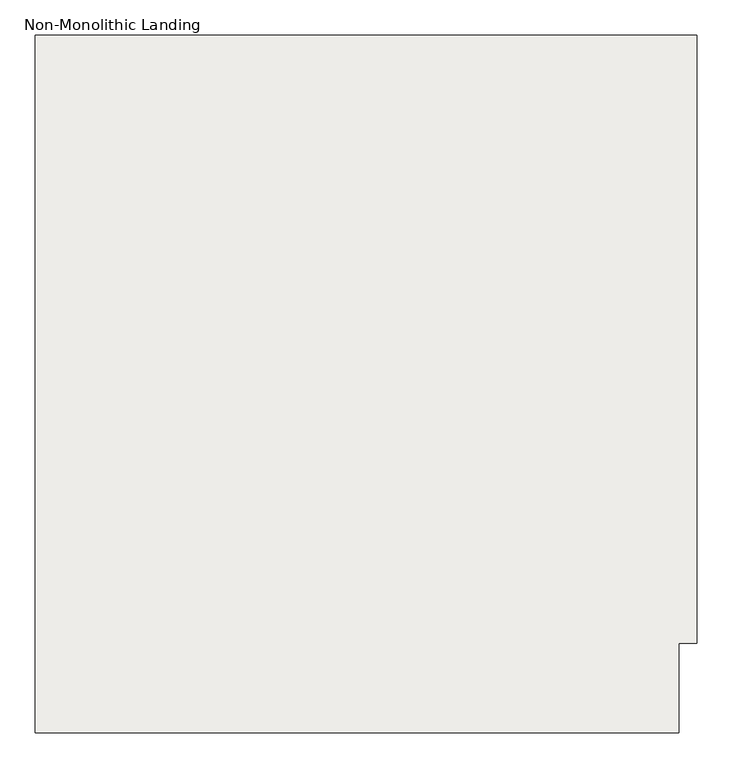
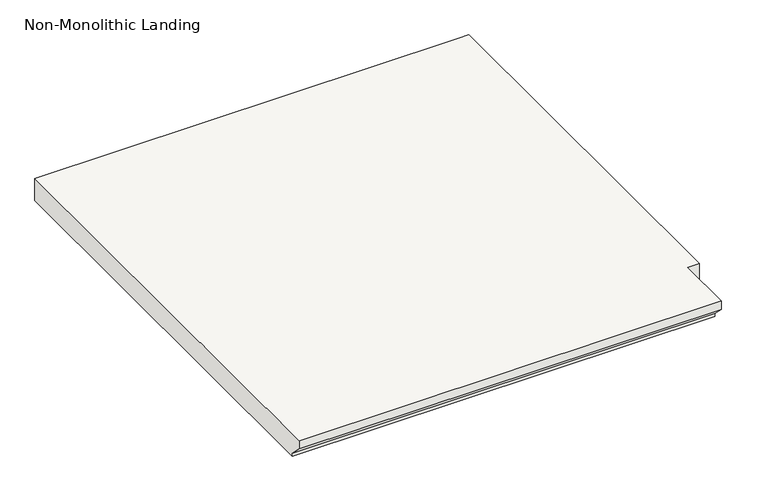
"""IFC4 building model written with IfcOpenShell, lengths in millimetres: slab geometry, Non-Monolithic Landing."""

from ifc_helpers import new_model, si_unit, origin, place, context, project, spatial, faceted_brep, source, transform, mapped, element, save


def non_monolithic_landing_17065b0a(model_context):
    return source(origin(), model_context, "Body", "Brep", [
        faceted_brep([(4429.2597674, 334.5758265, 2182.2833333), (4429.2597674, 334.5758265, 2201.3333333), (3514.8597674, 334.5758265, 2201.3333333), (3514.8597674, 334.5758265, 2182.2833333), (4429.2597674, 359.9758265, 2156.8833333), (3514.8597674, 359.9758265, 2156.8833333), (4429.2597674, 461.5758265, 2201.3333333), (4454.6597674, 461.5758265, 2201.3333333), (4454.6597674, 1325.1758265, 2201.3333333), (4429.2597674, 1325.1758265, 2201.3333333), (3514.8597674, 1325.1758265, 2201.3333333), (4429.2597674, 359.9758265, 2150.5333333), (3514.8597674, 359.9758265, 2150.5333333), (3514.8597674, 1325.1758265, 2150.5333333), (4429.2597674, 1325.1758265, 2150.5333333), (4454.6597674, 1325.1758265, 2150.5333333), (4454.6597674, 461.5758265, 2150.5333333), (4429.2597674, 461.5758265, 2150.5333333)], [[[0, 1, 2, 3]], [[4, 0, 3, 5]], [[6, 7, 8, 9, 10, 2, 1]], [[11, 12, 13, 14, 15, 16, 17]], [[12, 11, 4, 5]], [[6, 1, 0, 4, 11, 17]], [[7, 6, 17, 16]], [[8, 7, 16, 15]], [[9, 8, 15, 14]], [[10, 9, 14, 13]], [[2, 10, 13, 12, 5, 3]]]),
    ])


if __name__ == "__main__":
    model = new_model("IFC4")
    model_context = context("Model", 3, world=origin())
    ifc_project = project(units=[si_unit("LENGTHUNIT", "METRE", prefix="MILLI")], contexts=[model_context])
    site = spatial("IfcSite", under=ifc_project)
    building = spatial("IfcBuilding", under=site)
    placement = place(None, origin())
    non_monolithic_landing_shape = non_monolithic_landing_17065b0a(model_context)
    element("IfcSlab", 1, ObjectType="Non-Monolithic Landing", at=placement, inside=building, context=model_context, shape_type="MappedRepresentation", body=[
        mapped(non_monolithic_landing_shape, transform((0.0, 0.0, 0.0), x_axis=(1.0, 0.0, 0.0), y_axis=(0.0, 1.0, 0.0), z_axis=(0.0, 0.0, 1.0))),
    ])
    save(model, "model.ifc")
